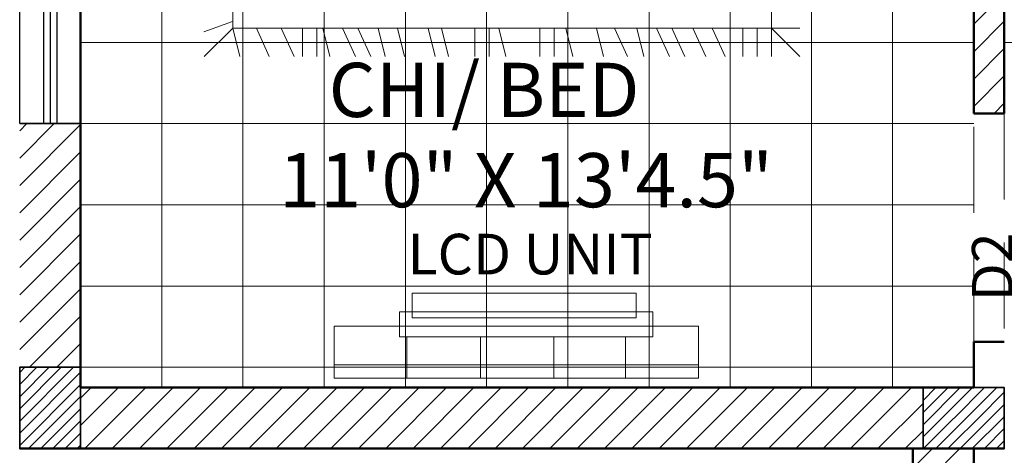
# Model space of a CAD drawing. Units: millimetres. Extents: x 225995 to 227247, y 225507 to 226008.
# Tile 13 of 23: x 226749 to 226894, y 225691 to 225755. Entities that reach past the tile are written whole.
import ezdxf

# ---------------------------------------------------------------- set-up
doc = ezdxf.new("R2010")
doc.units = ezdxf.units.MM
doc.linetypes.add('DASHED', pattern=[19.05, 12.7, -6.35])
for name, color, linetype, lineweight in [('A-ANNO-TEXT', 3, 'Continuous', 18), ('A-AREA-IDEN', 30, 'Continuous', 18), ('A-COLS', 40, 'Continuous', 35), ('A-FLOR-PATT', 8, 'Continuous', 13), ('A-FURN', 9, 'Continuous', 18), ('A-GLAZ', 4, 'Continuous', 25), ('A-WALL', 7, 'Continuous', 50), ('A-WALL-OVHD', 1, 'DASHED', 18), ('A-WALL-PATT', 8, 'Continuous', 13)]:
    doc.layers.add(name, color=color, linetype=linetype, lineweight=lineweight)
doc.styles.get("Standard").update_dxf_attribs({"font": 'arial.ttf'})
pattern_1 = [(45, (502.0463, 0.931), (-0.898025612, 0.898025612), [])]

# ---------------------------------------------------------------- blocks, each defined once
blk = doc.blocks.new('A$C6D2A2628')
for p, q in [((0.1019, 0.9267), (0.1019, 0.1)), ((1.9932, 0.1), (1.9932, 0.9267)), ((0, 0.0863), (0.1015, 0.1229)), ((0.1019, 0.1), (0.0019, 0)), ((0.1019, 0.1), (1.9932, 0.1)), ((0.1019, 0.1), (0.1266, 0)), ((0.1851, 0.1), (0.2305, 0)), ((0.2725, 0.1), (0.3179, 0)), ((0.3469, 0.1), (0.3469, 0)), ((0.3969, 0.1), (0.3969, 0)), ((0.4179, 0.1), (0.4426, 0)), ((0.4876, 0.1), (0.533, 0)), ((0.5414, 0.1), (0.5868, 0)), ((0.6128, 0.1), (0.6376, 0)), ((0.6801, 0.1), (0.7048, 0)), ((0.7876, 0.1), (0.8124, 0)), ((0.8347, 0.1), (0.8594, 0)), ((0.952, 0.1), (0.952, 0)), ((1.002, 0.1), (1.002, 0)), ((1.0364, 0.1), (1.0611, 0)), ((1.1805, 0.1), (1.1805, 0)), ((1.2305, 0.1), (1.2305, 0)), ((1.2717, 0.1), (1.2964, 0)), ((1.3792, 0.1), (1.404, 0)), ((1.4422, 0.1), (1.4876, 0)), ((1.5204, 0.1), (1.5451, 0)), ((1.5901, 0.1), (1.6355, 0)), ((1.6439, 0.1), (1.6893, 0)), ((1.7179, 0.1), (1.7633, 0)), ((1.7851, 0.1), (1.8305, 0)), ((1.8932, 0.1), (1.8932, 0)), ((1.9432, 0.1), (1.9432, 0)), ((1.9932, 0.1), (2.0932, 0.1)), ((1.9932, 0.1), (1.9932, 0)), ((1.9932, 0.1), (2.0932, 0))]:
    blk.add_line(p, q)

msp = doc.modelspace()

# ---------------------------------------------------------------- hatches: boundary and pattern name
at = {"layer": 'A-WALL-PATT'}
h = msp.add_hatch(dxfattribs=at)
h.set_pattern_fill('ANSI31', color=256, scale=0.9)
h.paths.add_polyline_path([(226894.42, 225809.84), (226889.92, 225809.84), (226889.92, 225741.2), (226894.42, 225741.2)])
h = msp.add_hatch(dxfattribs=at)
h.set_pattern_fill('ANSI31', color=256, scale=0.9)
h.paths.add_polyline_path([(226757.92, 225739.7), (226748.92, 225739.7), (226748.92, 225703.7), (226757.92, 225703.7)])
h = msp.add_hatch(dxfattribs=at)
h.set_pattern_fill('ANSI31', color=256, scale=0.4)
h.set_pattern_definition([(45, (646.0463, 120.931), (-0.898025612, 0.898025612), [])])
h.paths.add_polyline_path([(226757.92, 225703.7), (226748.92, 225703.7), (226748.92, 225691.7), (226757.92, 225691.7)])
h = msp.add_hatch(dxfattribs=at)
h.set_pattern_fill('ANSI31', color=256, scale=0.9)
h.paths.add_polyline_path([(226882.42, 225700.7), (226757.92, 225700.7), (226757.92, 225691.7), (226882.42, 225691.7)])
h = msp.add_hatch(dxfattribs=at)
h.set_pattern_fill('ANSI31', color=256, scale=0.4)
h.set_pattern_definition(pattern_1)
h.paths.add_polyline_path([(226886.92, 225700.7), (226882.42, 225700.7), (226882.42, 225696.2), (226886.92, 225696.2)])
h = msp.add_hatch(dxfattribs=at)
h.set_pattern_fill('ANSI31', color=256, scale=0.4)
h.set_pattern_definition(pattern_1)
h.paths.add_polyline_path([(226894.42, 225700.7), (226886.92, 225700.7), (226886.92, 225696.2), (226894.42, 225696.2)])
h = msp.add_hatch(dxfattribs=at)
h.set_pattern_fill('ANSI31', color=256, scale=0.4)
h.set_pattern_definition(pattern_1)
h.paths.add_polyline_path([(226886.92, 225696.2), (226882.42, 225696.2), (226882.42, 225691.7), (226886.92, 225691.7)])
h = msp.add_hatch(dxfattribs=at)
h.set_pattern_fill('ANSI31', color=256, scale=0.4)
h.set_pattern_definition(pattern_1)
h.paths.add_polyline_path([(226894.42, 225696.2), (226886.92, 225696.2), (226886.92, 225691.7), (226894.42, 225691.7)])
h = msp.add_hatch(dxfattribs=at)
h.set_pattern_fill('ANSI31', color=256, scale=0.9)
h.paths.add_polyline_path([(226889.92, 225691.7), (226882.42, 225691.7), (226880.92, 225691.7), (226880.92, 225673.56), (226889.92, 225673.56)])

# ---------------------------------------------------------------- linework, layer by layer
at = {"layer": 'A-COLS'}
msp.add_line((226757.92, 225739.7), (226748.92, 225739.7), dxfattribs=at)
for points in [[(226757.92, 225691.7), (226748.92, 225691.7), (226748.92, 225703.7), (226757.92, 225703.7)], [(226882.42, 225691.7), (226882.42, 225700.7), (226894.42, 225700.7), (226894.42, 225691.7)]]:
    msp.add_lwpolyline(points, close=True, dxfattribs=at)
at = {"layer": 'A-FLOR-PATT'}
for p, q in [((226769.92, 225700.7), (226769.92, 225925.7)), ((226781.92, 225700.7), (226781.92, 225925.7)), ((226793.92, 225700.7), (226793.92, 225925.7)), ((226805.92, 225861.2), (226805.92, 225700.7)), ((226817.92, 225861.2), (226817.92, 225700.7)), ((226829.92, 225861.2), (226829.92, 225700.7)), ((226841.92, 225861.2), (226841.92, 225700.7)), ((226853.92, 225861.2), (226853.92, 225700.7)), ((226865.92, 225861.2), (226865.92, 225700.7)), ((226877.92, 225861.2), (226877.92, 225700.7)), ((226757.92, 225751.7), (226889.92, 225751.7)), ((226894.42, 225751.7), (227026.42, 225751.7)), ((226757.92, 225739.7), (226889.92, 225739.7)), ((226757.92, 225727.7), (226889.92, 225727.7)), ((226757.92, 225715.7), (226889.92, 225715.7)), ((226757.92, 225703.7), (226889.92, 225703.7))]:
    msp.add_line(p, q, dxfattribs=at)
at = {"layer": 'A-FURN'}
for p, q in [((226757.92, 225691.7), (226757.92, 225809.85)), ((226806.11, 225708.2), (226806.11, 225702.1)), ((226817.01, 225708.2), (226817.01, 225705.04)), ((226827.87, 225708.2), (226827.87, 225702.1)), ((226838.44, 225708.2), (226838.44, 225702.1)), ((226795.39, 225704.05), (226849.21, 225704.05)), ((226817.01, 225705.04), (226817.01, 225702.1))]:
    msp.add_line(p, q, dxfattribs=at)
for points in [[(226806.93, 225714.67), (226840.02, 225714.67), (226840.02, 225711.01), (226806.93, 225711.01)], [(226805.05, 225711.9), (226842.47, 225711.9), (226842.47, 225708.2), (226805.05, 225708.2)], [(226795.39, 225709.79), (226849.21, 225709.79), (226849.21, 225702.1), (226795.39, 225702.1)]]:
    msp.add_lwpolyline(points, close=True, dxfattribs=at)
at = {"layer": 'A-GLAZ'}
for p, q in [((226752.42, 225787.7), (226752.42, 225739.7)), ((226753.42, 225787.7), (226753.42, 225739.7)), ((226754.42, 225787.7), (226754.42, 225739.7))]:
    msp.add_line(p, q, dxfattribs=at)
msp.add_lwpolyline([(226748.92, 225787.7), (226757.92, 225787.7), (226757.92, 225739.7), (226748.92, 225739.7)], close=True, dxfattribs=at)
at = {"layer": 'A-WALL'}
for p, q in [((226889.92, 225741.2), (226889.92, 225934.7)), ((226889.92, 225741.2), (226889.92, 225925.7)), ((226894.42, 225741.2), (226894.42, 225925.7)), ((226894.42, 225925.7), (226894.42, 225741.2)), ((226757.92, 225861.2), (226757.92, 225700.7)), ((226889.92, 225741.2), (226894.42, 225741.2)), ((226894.42, 225741.2), (226889.92, 225741.2)), ((226889.92, 225707.45), (226894.42, 225707.45)), ((226889.92, 225700.7), (226889.92, 225707.45)), ((226889.92, 225700.7), (226889.92, 225707.45)), ((226889.92, 225707.45), (226894.42, 225707.45)), ((226757.92, 225700.7), (226889.92, 225700.7)), ((226757.92, 225700.7), (226889.92, 225700.7)), ((226748.92, 225691.7), (226889.92, 225691.7)), ((226880.92, 225691.7), (226748.92, 225691.7)), ((226880.92, 225643.56), (226880.92, 225691.7)), ((226880.92, 225643.7), (226880.92, 225691.7)), ((226889.92, 225643.56), (226889.92, 225691.7)), ((226894.42, 225691.7), (226889.92, 225691.7)), ((226889.92, 225691.7), (226889.92, 225643.7))]:
    msp.add_line(p, q, dxfattribs=at)
at = {"layer": 'A-WALL-OVHD'}
msp.add_lwpolyline([(226889.92, 225741.2), (226894.42, 225741.2), (226894.42, 225707.45), (226889.92, 225707.45)], close=True, dxfattribs=at)

# ---------------------------------------------------------------- block references
at = {"layer": 'A-FURN', "xscale": 42.09102840542158, "yscale": 42.09102840542158, "zscale": 42.09102840542158}
msp.add_blockref('A$C6D2A2628', (226776.11, 225749.61), dxfattribs=at)

# ---------------------------------------------------------------- texts
at = {"layer": 'A-ANNO-TEXT', "insert": (226800.73, 225723.42), "char_height": 6, "attachment_point": 1}
msp.add_mtext_dynamic_manual_height_columns('   LCD UNIT', width=85.4795, gutter_width=12.5, heights=[0], dxfattribs=at)
at = {"layer": 'A-ANNO-TEXT', "insert": (226889.64, 225713.45), "char_height": 6, "attachment_point": 1, "rotation": 90}
msp.add_mtext_dynamic_manual_height_columns('D2', width=8.157, gutter_width=12.5, heights=[0], dxfattribs=at)
at = {"layer": 'A-AREA-IDEN', "insert": (226775.02, 225748.68), "char_height": 8, "attachment_point": 1}
msp.add_mtext_dynamic_manual_height_columns('        CHI/ BED\\P     11\'0" X 13\'4.5"', width=93.9568, gutter_width=12.5, heights=[0], dxfattribs=at)

doc.saveas('drawing.dxf')
